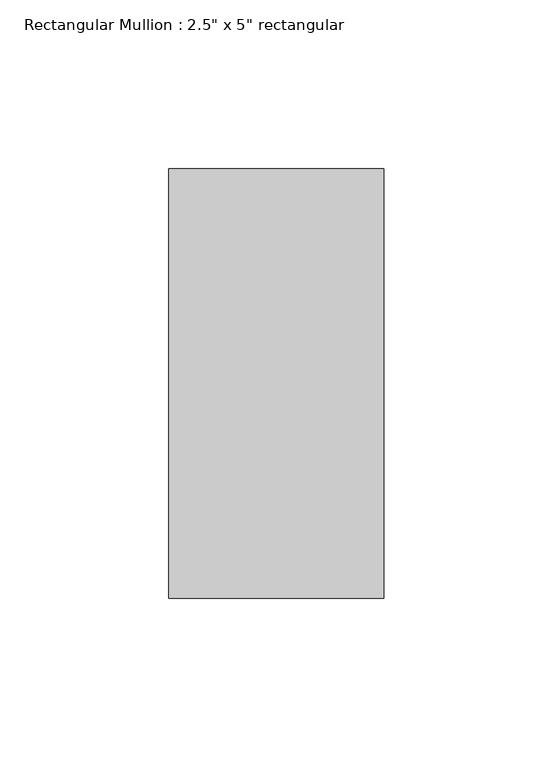
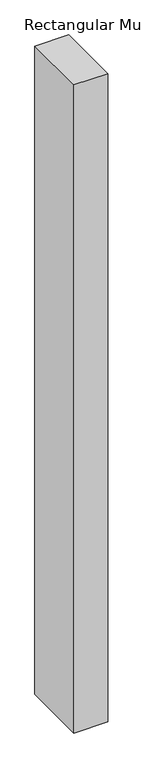
"""IFC4 building model written with IfcOpenShell, lengths in millimetres: member geometry."""

from ifc_helpers import new_model, si_unit, frame, origin, place, context, project, spatial, polyline, outline, extrude, source, transform, mapped, element, save


def member_bb4f9a93(model_context):
    return source(origin(), model_context, "Body", "SweptSolid", [
        extrude(outline(polyline([(31.75, 63.5), (31.75, -63.5), (-31.75, -63.5), (-31.75, 63.5), (31.75, 63.5)])), frame((0.0, 0.0, -1288.0294817), z_axis=(0.0, 0.0, 1.0), x_axis=(1.0, 0.0, 0.0)), (0.0, 0.0, 1.0), 1288.0294817),
    ])


if __name__ == "__main__":
    model = new_model("IFC4")
    model_context = context("Model", 3, world=origin())
    ifc_project = project(units=[si_unit("LENGTHUNIT", "METRE", prefix="MILLI")], contexts=[model_context])
    site = spatial("IfcSite", under=ifc_project)
    building = spatial("IfcBuilding", under=site)
    placement = place(None, origin())
    member_shape = member_bb4f9a93(model_context)
    element("IfcMember", 1, ObjectType="Rectangular Mullion : 2.5\" x 5\" rectangular", at=placement, inside=building, context=model_context, shape_type="MappedRepresentation", body=[
        mapped(member_shape, transform((0.0, 0.0, 0.0), x_axis=(1.0, 0.0, 0.0), y_axis=(0.0, 1.0, 0.0), z_axis=(0.0, 0.0, 1.0))),
    ])
    save(model, "model.ifc")

# Revit data of these elements
# Type "Rectangular Mullion : 2.5\" x 5\" rectangular"
#   built-in parameter 1007304 = 0.416667 (stored number, unit not read)
#   built-in parameter 1007301 = 0.104167 (stored number, unit not read)
#   built-in parameter 1007300 = 0.104167 (stored number, unit not read)
# Element 1 (IfcMember, "Rectangular Mullion : 2.5\" x 5\" rectangular")
#   Materials on its faces: "Aluminum"
# Materials
#   "Aluminum": class "Metal", colour RGB 247 247 247, transparency 0, Description = "Aluminum 6061", Cost = 0
